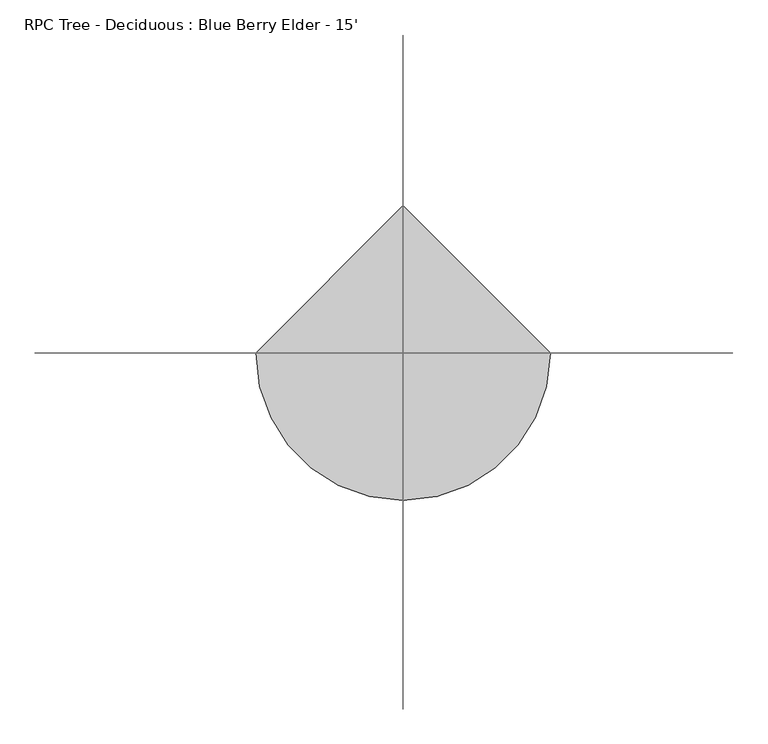
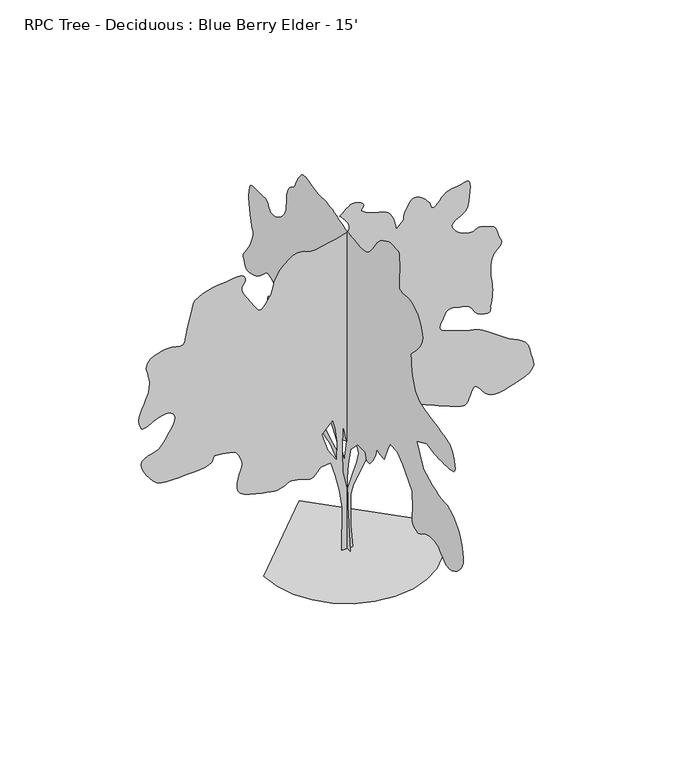
"""IFC4 building model written with IfcOpenShell, lengths in millimetres: geographic element geometry, RPC Tree - Deciduous : Blue Berry Elder - 15'."""

from ifc_helpers import new_model, si_unit, origin, place, context, project, spatial, triangles, source, transform, mapped, element, save


def rpc_tree_deciduous_blue_berry_elder_15_4a646840(model_context):
    return source(origin(), model_context, "Body", "Tessellation", [
        triangles([(-0.0006962, 27.8334278, 0.0019603), (-0.0006962, -29.6324096, 0.0019603), (-0.0006962, -7.2846616, 268.1759455), (-0.0006962, -0.8995193, 430.9958582), (-0.0006962, -10.4771573, 523.5799235), (-0.0006962, -36.0175667, 628.9336309), (-0.0006962, -106.2537161, 699.1706228), (-0.0006962, -179.6824553, 699.1706228), (-0.0006962, -195.6453436, 654.4740051), (-0.0006962, -227.5699575, 657.6673422), (-0.0006962, -262.6890348, 699.1706228), (-0.0006962, -285.0361446, 743.8660051), (-0.0006962, -297.8069494, 788.5613874), (-0.0006962, -332.9248458, 775.791818), (-0.0006962, -371.2348257, 772.598481), (-0.0006962, -406.3527403, 852.4130133), (-0.0006962, -431.8931508, 900.3004972), (-0.0006962, -502.1301064, 897.1083956), (-0.0006962, -556.4030291, 852.4130133), (-0.0006962, -655.3724968, 747.0581068), (-0.0006962, -658.5645985, 641.7044357), (-0.0006962, -657.5866785, 629.1849237), (-0.0006962, -655.4376818, 614.2651222), (-0.0006962, -653.2875223, 598.0604064), (-0.0006962, -652.3096024, 581.6873869), (-0.0006962, -653.6774694, 566.2649998), (-0.0006962, -658.5645985, 552.9086566), (-0.0006962, -668.1421389, 542.7349317), (-0.0006962, -680.1305786, 535.3822918), (-0.0006962, -691.7279085, 530.0388316), (-0.0006962, -703.3252384, 527.1537243), (-0.0006962, -715.3136782, 527.1726912), (-0.0006962, -728.084483, 530.5425799), (-0.0006962, -742.0263645, 537.709112), (-0.0006962, -757.5340662, 549.1203341), (-0.0006962, -776.7637791, 561.2296967), (-0.0006962, -800.3495487, 570.1552783), (-0.0006962, -826.3925085, 575.8425038), (-0.0006962, -852.9937918, 578.234509), (-0.0006962, -878.2544592, 577.276755), (-0.0006962, -900.2768068, 572.9111784), (-0.0006962, -917.1607327, 565.0832405), (-0.0006962, -931.1227438, 553.3365738), (-0.0006962, -945.9773603, 538.7427335), (-0.0006962, -962.2282579, 523.5337054), (-0.0006962, -980.3793303, 509.9438373), (-0.0006962, -1000.9306194, 500.208712), (-0.0006962, -1024.3860191, 496.5590438), (-0.0006962, -1051.248115, 501.231651), (-0.0006962, -1078.7241268, 513.6764583), (-0.0006962, -1103.3530014, 530.8116405), (-0.0006962, -1124.629755, 551.0749386), (-0.0006962, -1142.0542002, 572.901695), (-0.0006962, -1155.1225159, 594.7284513), (-0.0006962, -1163.3309538, 614.990514), (-0.0006962, -1166.1792538, 632.1268953), (-0.0006962, -1164.3550192, 650.8540226), (-0.0006962, -1159.4039406, 675.2209219), (-0.0006962, -1152.1058395, 702.6602354), (-0.0006962, -1143.2454065, 730.6021345), (-0.0006962, -1133.6027538, 756.4779533), (-0.0006962, -1123.9600285, 777.7180086), (-0.0006962, -1115.0985054, 791.7534891), (-0.0006962, -1104.8050203, 803.3887527), (-0.0006962, -1090.6011635, 817.9825567), (-0.0006962, -1072.8792801, 833.8068089), (-0.0006962, -1052.0304073, 849.12724), (-0.0006962, -1028.4446377, 862.2133598), (-0.0006962, -1002.513081, 871.3344601), (-0.0006962, -974.6269197, 874.7601231), (-0.0006962, -945.6146645, 877.0869432), (-0.0006962, -916.0998236, 883.6026793), (-0.0006962, -886.1665489, 893.6081005), (-0.0006962, -855.8979023, 906.4061565), (-0.0006962, -825.3778902, 921.2987068), (-0.0006962, -794.6895744, 937.5875381), (-0.0006962, -763.9183422, 954.57342), (-0.0006962, -696.8746147, 1079.0832619), (-0.0006962, -799.0361841, 1126.9719812), (-0.0006962, -812.7931932, 1122.8943958), (-0.0006962, -826.9970501, 1118.9851868), (-0.0006962, -842.0946751, 1115.4114223), (-0.0006962, -858.5316805, 1112.3402435), (-0.0006962, -876.7562222, 1109.9387186), (-0.0006962, -897.2150751, 1108.3752966), (-0.0006962, -920.353997, 1107.8158104), (-0.0006962, -946.7881393, 1107.7138544), (-0.0006962, -975.4554302, 1107.7790394), (-0.0006962, -1004.2910975, 1108.5696888), (-0.0006962, -1031.2277527, 1110.6463789), (-0.0006962, -1054.1983709, 1114.5638723), (-0.0006962, -1071.1391973, 1120.8841261), (-0.0006962, -1079.9805908, 1130.1640829), (-0.0006962, -1081.6756182, 1144.7863735), (-0.0006962, -1079.0690912, 1165.0496716), (-0.0006962, -1072.9444651, 1188.3805876), (-0.0006962, -1064.0828693, 1212.21765), (-0.0006962, -1053.2679045, 1233.9922657), (-0.0006962, -1041.2793921, 1251.1322079), (-0.0006962, -1028.8997698, 1261.0534046), (-0.0006962, -1016.4087444, 1266.0318798), (-0.0006962, -1002.85681, 1270.3346695), (-0.0006962, -987.1831301, 1274.4595631), (-0.0006962, -968.3256329, 1278.928331), (-0.0006962, -945.2234819, 1284.2386173), (-0.0006962, -916.8157682, 1290.8764389), (-0.0006962, -882.0428181, 1299.3634209), (-0.0006962, -844.7746714, 1307.803022), (-0.0006962, -809.8523844, 1314.8438713), (-0.0006962, -777.6658316, 1321.8136494), (-0.0006962, -748.6073582, 1330.0872723), (-0.0006962, -723.066984, 1340.9805027), (-0.0006962, -701.4358189, 1355.8327938), (-0.0006962, -684.1050453, 1375.9953712), (-0.0006962, -670.8233706, 1400.3658314), (-0.0006962, -660.7242777, 1426.7512848), (-0.0006962, -653.2780025, 1454.8200657), (-0.0006962, -647.9534729, 1484.2163818), (-0.0006962, -644.2208519, 1514.6319672), (-0.0006962, -641.5503027, 1545.7114655), (-0.0006962, -639.4095903, 1577.1227749), (-0.0006962, -663.2087191, 1601.7422024), (-0.0006962, -686.1438017, 1626.3023312), (-0.0006962, -707.3458506, 1650.7557804), (-0.0006962, -725.952055, 1675.0432514), (-0.0006962, -741.0958981, 1699.0936729), (-0.0006962, -751.9120256, 1722.8833546), (-0.0006962, -757.5340662, 1746.3293072), (-0.0006962, -755.6351995, 1772.2525795), (-0.0006962, -745.4709217, 1801.6369778), (-0.0006962, -728.5491348, 1831.6851437), (-0.0006962, -706.3786131, 1859.6235546), (-0.0006962, -680.4660233, 1882.6427891), (-0.0006962, -652.3191221, 1897.9453434), (-0.0006962, -623.4466839, 1902.7578403), (-0.0006962, -596.6771333, 1901.3236256), (-0.0006962, -573.873656, 1900.2094494), (-0.0006962, -555.0908635, 1900.1619232), (-0.0006962, -540.3844211, 1901.9044041), (-0.0006962, -529.8112292, 1906.1598129), (-0.0006962, -523.4258268, 1913.6510708), (-0.0006962, -521.2851145, 1925.1133072), (-0.0006962, -522.0946944, 1946.4848225), (-0.0006962, -523.853744, 1979.579314), (-0.0006962, -525.5570558, 2018.9324352), (-0.0006962, -526.1995311, 2059.0679214), (-0.0006962, -524.7747634, 2094.5093628), (-0.0006962, -520.2799796, 2119.7925579), (-0.0006962, -511.7076104, 2129.4293243), (-0.0006962, -499.1608472, 2130.0813194), (-0.0006962, -484.0442917, 2131.5155342), (-0.0006962, -467.309739, 2132.949749), (-0.0006962, -449.9042971, 2133.6017441), (-0.0006962, -432.7773992, 2132.6890091), (-0.0006962, -416.879714, 2129.4293243), (-0.0006962, -403.1606386, 2123.0522427), (-0.0006962, -390.1302567, 2115.4660778), (-0.0006962, -375.9263998, 2108.5675163), (-0.0006962, -360.9402143, 2101.43176), (-0.0006962, -345.5640452, 2093.1818275), (-0.0006962, -330.1879126, 2082.9286743), (-0.0006962, -315.2028897, 2069.7714832), (-0.0006962, -300.999051, 2052.8092918), (-0.0006962, -286.7584414, 2032.3385937), (-0.0006962, -271.5126786, 2010.2557846), (-0.0006962, -255.4288675, 1988.0545235), (-0.0006962, -238.6741671, 1967.2518688), (-0.0006962, -221.4180801, 1949.3533974), (-0.0006962, -203.8265303, 1935.8642498), (-0.0006962, -186.0678577, 1928.3017754), (-0.0006962, -167.8895705, 1925.4688087), (-0.0006962, -148.9301446, 1924.816959), (-0.0006962, -129.188399, 1925.7888474), (-0.0006962, -108.6643338, 1927.8157585), (-0.0006962, -87.3590209, 1930.3523769), (-0.0006962, -65.2717381, 1932.829842), (-0.0006962, -42.4027261, 1934.6907749), (-0.0006962, -15.4102944, 1938.1638187), (-0.0006962, 16.7757986, 1944.9439281), (-0.0006962, 50.749019, 1953.6205788), (-0.0006962, 83.1026037, 1962.7950188), (-0.0006962, 110.4301236, 1971.0805595), (-0.0006962, 129.3247097, 1977.0783039), (-0.0006962, 136.3798205, 1979.3778728), (-0.0006962, 140.2617874, 1980.586956), (-0.0006962, 151.0115855, 1983.5857555), (-0.0006962, 167.2909697, 1987.4262188), (-0.0006962, 187.7581434, 1991.14823), (-0.0006962, 211.0748524, 1993.8034458), (-0.0006962, 235.8981192, 1994.4552956), (-0.0006962, 260.8897079, 1992.1557266), (-0.0006962, 288.430941, 1991.7053181), (-0.0006962, 320.1611627, 1996.7904728), (-0.0006962, 353.6219473, 2004.7203667), (-0.0006962, 386.3573401, 2012.8160934), (-0.0006962, 415.9100784, 2018.3990376), (-0.0006962, 439.8206466, 2018.7902927), (-0.0006962, 455.6353789, 2011.3108074), (-0.0006962, 466.5440154, 1998.4499645), (-0.0006962, 477.2286103, 1984.6288605), (-0.0006962, 487.4675202, 1970.0967533), (-0.0006962, 497.0355409, 1955.0547935), (-0.0006962, 505.7098297, 1939.7284035), (-0.0006962, 513.268707, 1924.3546326), (-0.0006962, 519.4858057, 1909.1468399), (-0.0006962, 526.9130776, 1896.1673996), (-0.0006962, 537.4685017, 1886.2698933), (-0.0006962, 549.9773312, 1877.8183743), (-0.0006962, 563.2696521, 1869.2010223), (-0.0006962, 576.1696641, 1858.7938087), (-0.0006962, 587.5061814, 1844.97285), (-0.0006962, 596.1069646, 1826.1378078), (-0.0006962, 601.3283755, 1809.8395294), (-0.0006962, 603.8697175, 1802.0873863), (-0.0006962, 604.5678944, 1798.9106907), (-0.0006962, 604.2609, 1796.3503819), (-0.0006962, 603.7855657, 1790.4473991), (-0.0006962, 603.9811569, 1777.2191368), (-0.0006962, 605.6844687, 1752.7063889), (-0.0006962, 608.6916615, 1724.7088245), (-0.0006962, 612.535722, 1702.6970867), (-0.0006962, 617.6634613, 1685.1897251), (-0.0006962, 624.522999, 1670.7642975), (-0.0006962, 633.5611828, 1657.962608), (-0.0006962, 645.2236977, 1645.3151241), (-0.0006962, 659.9585541, 1631.3992584), (-0.0006962, 676.6931431, 1617.5426914), (-0.0006962, 693.7642668, 1606.2109703), (-0.0006962, 710.7216619, 1597.5460922), (-0.0006962, 727.121969, 1591.7380165), (-0.0006962, 742.5171049, 1588.9524307), (-0.0006962, 756.4602219, 1589.3436859), (-0.0006962, 768.5043995, 1593.0892422), (-0.0006962, 777.4406273, 1600.4383575), (-0.0006962, 783.6944607, 1610.4662338), (-0.0006962, 789.2797302, 1621.5610508), (-0.0006962, 796.2044529, 1632.0986343), (-0.0006962, 806.4801338, 1640.4552464), (-0.0006962, 822.1170427, 1645.0187759), (-0.0006962, 845.1255947, 1644.1653397), (-0.0006962, 872.6667915, 1642.5058479), (-0.0006962, 899.7066381, 1643.8096928), (-0.0006962, 924.9578585, 1645.1728363), (-0.0006962, 947.13899, 1643.6793228), (-0.0006962, 964.9628294, 1636.436887), (-0.0006962, 977.1468967, 1620.5416363), (-0.0006962, 982.4050787, 1593.0892422), (-0.0006962, 983.5406199, 1565.7080647), (-0.0006962, 984.0621723, 1548.8288624), (-0.0006962, 983.7456945, 1537.7105003), (-0.0006962, 982.3683077, 1527.5994896), (-0.0006962, 979.7060429, 1513.7311501), (-0.0006962, 975.5360212, 1491.3876011), (-0.0006962, 969.6354366, 1455.8038719), (-0.0006962, 961.9189018, 1419.4496956), (-0.0006962, 953.6452789, 1394.8183502), (-0.0006962, 946.5984707, 1377.2279995), (-0.0006962, 942.5683388, 1361.9845985), (-0.0006962, 943.341184, 1344.3942478), (-0.0006962, 950.7033073, 1319.7630478), (-0.0006962, 966.4421722, 1283.4088715), (-0.0006962, 986.743404, 1245.2885239), (-0.0006962, 1005.7027845, 1216.9471579), (-0.0006962, 1021.9821688, 1196.0378237), (-0.0006962, 1034.2397055, 1180.2029617), (-0.0006962, 1041.1371769, 1167.1062321), (-0.0006962, 1041.3327318, 1154.401775), (-0.0006962, 1033.4858271, 1139.7415506), (-0.0006962, 1024.3362402, 1124.5610092), (-0.0006962, 1019.3199039, 1112.116202), (-0.0006962, 1015.1404352, 1102.7994741), (-0.0006962, 1008.5037764, 1097.0007729), (-0.0006962, 996.115797, 1095.1113533), (-0.0006962, 974.6802595, 1097.5223253), (-0.0006962, 940.9017254, 1104.6237087), (-0.0006962, 904.0438007, 1118.2964933), (-0.0006962, 874.3334049, 1137.777499), (-0.0006962, 849.9285719, 1159.492816), (-0.0006962, 828.9860275, 1179.8675171), (-0.0006962, 809.6639511, 1195.3266752), (-0.0006962, 790.1165977, 1202.2963806), (-0.0006962, 768.5043995, 1197.2112986), (-0.0006962, 747.6649738, 1185.1730799), (-0.0006962, 731.1805876, 1173.6409349), (-0.0006962, 718.3267937, 1162.5272964), (-0.0006962, 708.3771103, 1151.7490299), (-0.0006962, 700.6048376, 1141.2220562), (-0.0006962, 694.2846565, 1130.8622234), (-0.0006962, 688.6911026, 1120.5866152), (-0.0006962, 697.5798769, 1111.7345392), (-0.0006962, 706.4402372, 1103.1349188), (-0.0006962, 715.2460951, 1095.0367212), (-0.0006962, 723.9666384, 1087.6935648), (-0.0006962, 732.5768686, 1081.3544168), (-0.0006962, 741.0472818, 1076.2728956), (-0.0006962, 749.3493914, 1072.6978958), (-0.0006962, 758.2014673, 1071.0787359), (-0.0006962, 767.7789351, 1070.6875534), (-0.0006962, 777.2449997, 1070.0178268), (-0.0006962, 785.761631, 1067.5606367), (-0.0006962, 792.4907988, 1061.8082262), (-0.0006962, 796.5956354, 1051.2528385), (-0.0006962, 797.2380381, 1034.3878796), (-0.0006962, 795.1151299, 1015.5861202), (-0.0006962, 791.5970306, 999.2972162), (-0.0006962, 786.8497913, 984.1261219), (-0.0006962, 781.041643, 968.6753208), (-0.0006962, 774.3409618, 951.5484592), (-0.0006962, 766.9124908, 931.3515089), (-0.0006962, 758.9268591, 906.6858633), (-0.0006962, 750.6804874, 878.9206249), (-0.0006962, 742.9924393, 851.0996487), (-0.0006962, 736.8120752, 824.3407442), (-0.0006962, 733.088974, 799.7580877), (-0.0006962, 732.7724962, 778.4718143), (-0.0006962, 736.8120752, 761.5974083), (-0.0006962, 746.1572897, 750.2513712), (-0.0006962, 758.1919476, 742.6925303), (-0.0006962, 769.7240925, 736.3083269), (-0.0006962, 780.8378036, 730.8996454), (-0.0006962, 791.6159975, 726.2744917), (-0.0006962, 802.1429712, 722.23484), (-0.0006962, 812.502804, 718.5863708), (-0.0006962, 822.7784849, 715.1322939), (-0.0006962, 833.6396679, 719.758683), (-0.0006962, 843.9995007, 723.4071522), (-0.0006962, 853.3541622, 725.1010168), (-0.0006962, 861.1999043, 723.8635197), (-0.0006962, 867.0364666, 718.7167408), (-0.0006962, 870.3589382, 708.6829056), (-0.0006962, 870.6659689, 692.7851841), (-0.0006962, 867.9017481, 675.8633972), (-0.0006962, 862.6246719, 662.9633852), (-0.0006962, 855.2530289, 653.4131687), (-0.0006962, 846.205398, 646.5441113), (-0.0006962, 835.9013031, 641.6854689), (-0.0006962, 824.7603407, 638.1673697), (-0.0006962, 813.1997818, 635.318997), (-0.0006962, 807.717631, 631.8471886), (-0.0006962, 802.1797422, 628.0683495), (-0.0006962, 796.5303778, 623.6755217), (-0.0006962, 790.7127823, 618.3604391), (-0.0006962, 784.672308, 611.8173792), (-0.0006962, 778.3521269, 603.7381485), (-0.0006962, 771.6976639, 593.8157164), (-0.0006962, 762.5291101, 583.2425609), (-0.0006962, 749.1727306, 573.3390956), (-0.0006962, 732.3255758, 563.9939175), (-0.0006962, 712.6857862, 555.0955871), (-0.0006962, 690.9526651, 546.5327376), (-0.0006962, 667.823263, 538.1927307), (-0.0006962, 643.9956476, 529.9653259), (-0.0006962, 567.3744887, 574.6607446), (-0.0006962, 490.7532935, 517.1945211), (-0.0006962, 480.5049002, 515.8633887), (-0.0006962, 470.3406587, 514.7562979), (-0.0006962, 460.3447208, 514.094892), (-0.0006962, 450.5989131, 514.1043755), (-0.0006962, 441.1897127, 515.0075907), (-0.0006962, 432.1977834, 517.0274165), (-0.0006962, 423.7096024, 520.3878219), (-0.0006962, 415.83541, 524.8363875), (-0.0006962, 408.406939, 529.7875388), (-0.0006962, 401.0910338, 534.9626953), (-0.0006962, 393.5523225, 540.0821503), (-0.0006962, 385.4541249, 544.8661606), (-0.0006962, 376.4633583, 549.0361822), (-0.0006962, 366.2434153, 552.3124357), (-0.0006962, 354.7397206, 554.8632611), (-0.0006962, 342.2297284, 557.0786782), (-0.0006962, 328.8828323, 559.0143159), (-0.0006962, 314.8650833, 560.7271111), (-0.0006962, 300.3447487, 562.2716025), (-0.0006962, 285.4901321, 563.7058537), (-0.0006962, 270.4672119, 565.0832405), (-0.0006962, 171.497726, 536.3495293), (-0.0006962, 88.491846, 475.6912405), (-0.0006962, 43.7962048, 402.263346), (-0.0006962, 21.4482684, 261.7905613), (-0.0006523, 31.0258883, 520.3878219), (-0.0006523, 78.9142239, 622.5494276), (-0.0006523, 2.2929818, 654.4740051), (-0.0006582, 145.9573246, 555.5057364), (-0.0006582, 222.5785107, 606.5865211), (-0.0006582, 283.2368176, 609.7786228), (-0.0006582, 334.3176023, 638.5110987), (-0.0006582, 331.5629013, 639.9916042), (-0.0006582, 328.6955618, 642.1418364), (-0.0006582, 325.6065788, 645.6326117), (-0.0006582, 322.1809522, 651.1325666), (-0.0006582, 318.3084778, 659.314916), (-0.0006582, 313.878879, 670.847061), (-0.0006582, 308.7771918, 686.399818), (-0.0006582, 304.7008418, 701.7664673), (-0.0006582, 303.1373835, 712.7782225), (-0.0006582, 303.6672385, 720.1593126), (-0.0006582, 305.873154, 724.6363649), (-0.0006582, 309.336678, 726.9346985), (-0.0006582, 313.6359069, 727.7821758), (-0.0006582, 318.3558949, 727.9030987), (-0.0006582, 321.5479966, 766.2131149), (-0.0006582, 283.2368176, 791.7534891), (-0.0006582, 200.2314009, 721.5177326), (-0.0006582, 142.7652138, 654.4740051), (-0.0006582, 104.4544981, 600.2011188), (-0.0006582, 66.1439051, 514.0024195), (31.5943742, 0.0001246, 0.0), (-32.2567384, 0.0001246, 0.0), (-29.0642779, 0.0001077, 261.7893804), (-45.0270572, 0.0001014, 376.7205737), (-67.3747574, 9.51e-05, 472.4967771), (-96.1076148, 9.08e-05, 558.6954763), (-153.5730934, 9.08e-05, 552.3112367), (-163.1790477, 9.08e-05, 538.7676229), (-172.9521249, 9.29e-05, 526.0632022), (-183.0606648, 9.29e-05, 515.0336792), (-193.6717722, 9.29e-05, 506.5170479), (-204.952588, 9.51e-05, 501.3513748), (-217.0702713, 9.51e-05, 500.3734549), (-230.1942886, 9.29e-05, 504.4225536), (-244.1563361, 9.29e-05, 510.5187295), (-258.6209692, 9.29e-05, 515.2754886), (-273.504036, 9.29e-05, 518.9144743), (-288.7213484, 9.29e-05, 521.660891), (-304.1911527, 9.29e-05, 523.736382), (-319.8280798, 9.29e-05, 525.3650617), (-335.5491769, 9.29e-05, 526.7708625), (-348.5890423, 9.29e-05, 519.3245873), (-361.8802005, 9.29e-05, 512.3524475), (-375.675107, 9.29e-05, 506.3309401), (-390.2227292, 9.29e-05, 501.7330376), (-405.7754863, 9.51e-05, 499.0340381), (-422.5859064, 9.51e-05, 498.7080769), (-440.902848, 9.51e-05, 501.230452), (-464.5822892, 9.29e-05, 505.7999042), (-495.0738147, 9.29e-05, 511.5985691), (-529.0289005, 9.29e-05, 519.0732945), (-563.0954258, 9.29e-05, 528.6697655), (-593.9223959, 9.08e-05, 540.8348296), (-618.1589252, 9.08e-05, 556.0154074), (-632.455291, 8.87e-05, 574.6583465), (-637.0721603, 8.87e-05, 596.876249), (-635.7694782, 8.66e-05, 621.4387396), (-630.4449486, 8.45e-05, 646.7847942), (-622.9986734, 8.45e-05, 671.3472485), (-615.3295195, 8.24e-05, 693.565151), (-609.3352996, 8.24e-05, 711.8726818), (-606.9148441, 8.03e-05, 724.7086716), (-608.023134, 8.03e-05, 735.682493), (-611.0848658, 8.03e-05, 748.77806), (-615.7112549, 7.82e-05, 762.9913639), (-621.5098835, 7.82e-05, 777.3161436), (-628.0908772, 7.6e-05, 790.7471552), (-635.0618179, 7.6e-05, 802.2793001), (-642.0339214, 7.6e-05, 810.9073345), (-651.2013124, 7.6e-05, 817.0971457), (-664.5588547, 7.39e-05, 822.1134819), (-681.4048468, 7.39e-05, 826.1531336), (-701.0446363, 7.39e-05, 829.4104202), (-722.7777575, 7.39e-05, 832.0821321), (-745.9071596, 7.39e-05, 834.3627342), (-769.734775, 7.39e-05, 836.4477087), (-773.4400721, 7.39e-05, 824.2174232), (-778.8475908, 7.6e-05, 812.4897234), (-787.6617331, 7.6e-05, 801.7671947), (-801.5870459, 7.6e-05, 792.5524229), (-822.3244429, 7.6e-05, 785.3479935), (-851.5785439, 7.82e-05, 780.6575821), (-891.0525152, 7.82e-05, 778.9815216), (-934.7890171, 7.82e-05, 777.8921986), (-975.5111681, 7.82e-05, 775.7420391), (-1012.9368633, 7.82e-05, 774.2070311), (-1046.7888668, 7.82e-05, 774.9609095), (-1076.7884892, 7.82e-05, 779.6797348), (-1102.6536255, 7.6e-05, 790.0394949), (-1124.1082026, 7.6e-05, 807.7152328), (-1143.5156662, 7.39e-05, 830.946591), (-1162.0839369, 7.39e-05, 855.9654127), (-1177.8050703, 7.18e-05, 881.4323175), (-1188.6650906, 6.97e-05, 906.0043642), (-1192.6596142, 6.76e-05, 928.343117), (-1187.776046, 6.76e-05, 947.1070152), (-1171.9969219, 6.76e-05, 960.9564606), (-1151.4171461, 6.55e-05, 969.659127), (-1133.2388226, 6.55e-05, 975.0678085), (-1117.127742, 6.55e-05, 978.9675705), (-1102.7472971, 6.55e-05, 983.1470392), (-1089.7631332, 6.55e-05, 989.3925882), (-1077.8398785, 6.34e-05, 999.4904457), (-1066.6420155, 6.34e-05, 1015.230546), (-1053.3888273, 6.13e-05, 1035.9584232), (-1037.2302933, 6.13e-05, 1059.0878981), (-1020.7363873, 5.91e-05, 1083.5021782), (-1006.4767925, 5.7e-05, 1108.083672), (-997.0202477, 5.7e-05, 1131.7168951), (-994.9352005, 5.49e-05, 1153.2828753), (-1002.791625, 5.49e-05, 1171.6650381), (-1017.218288, 5.28e-05, 1184.6396822), (-1032.9856396, 5.28e-05, 1191.4150681), (-1049.8695654, 5.28e-05, 1193.0271063), (-1067.6471867, 5.28e-05, 1190.5023331), (-1086.0956972, 5.28e-05, 1184.8826906), (-1104.9899654, 5.28e-05, 1177.1934071), (-1124.1082026, 5.49e-05, 1168.4729364), (-1137.7158749, 5.49e-05, 1161.0633596), (-1150.8777895, 5.49e-05, 1154.3532314), (-1163.144846, 5.49e-05, 1149.0381489), (-1174.0712139, 5.49e-05, 1145.8176332), (-1183.2125164, 5.49e-05, 1145.3896797), (-1190.1230684, 5.49e-05, 1148.4514114), (-1194.3427963, 5.49e-05, 1155.7021317), (-1197.5313372, 5.49e-05, 1164.6845776), (-1201.0518345, 5.49e-05, 1173.2201757), (-1204.0625519, 5.28e-05, 1182.4255005), (-1205.7338888, 5.28e-05, 1193.4182888), (-1205.2360268, 5.28e-05, 1207.3103914), (-1201.7156021, 5.07e-05, 1225.232626), (-1194.3427963, 4.86e-05, 1248.2873234), (-1184.4785002, 4.86e-05, 1272.8830605), (-1174.4445923, 4.65e-05, 1295.3688972), (-1164.8576048, 4.65e-05, 1316.72864), (-1156.3315264, 4.44e-05, 1337.9697853), (-1149.4815084, 4.22e-05, 1360.1236656), (-1144.9203043, 4.22e-05, 1384.1623146), (-1143.2632107, 4.01e-05, 1411.1048561), (-1145.1348261, 3.8e-05, 1436.9451393), (-1149.6296099, 3.8e-05, 1457.9255447), (-1155.0750624, 3.59e-05, 1475.4448242), (-1159.7938877, 3.59e-05, 1490.8898117), (-1162.1124235, 3.38e-05, 1505.6708862), (-1160.3522112, 3.38e-05, 1521.1750271), (-1152.8419138, 3.17e-05, 1538.8127586), (-1138.7032419, 3.17e-05, 1555.7038788), (-1119.4830488, 2.96e-05, 1568.4106613), (-1097.1347763, 2.96e-05, 1577.431041), (-1073.614119, 2.96e-05, 1583.2628071), (-1050.8758993, 2.96e-05, 1586.4158123), (-1030.8733412, 2.96e-05, 1587.3996185), (-1015.5624298, 2.96e-05, 1586.700388), (-1002.4289291, 2.96e-05, 1584.0807804), (-988.2902573, 2.96e-05, 1580.2403172), (-974.0958475, 2.96e-05, 1577.0636215), (-960.7952059, 2.96e-05, 1576.4590073), (-949.336603, 2.96e-05, 1580.3231609), (-940.6717976, 2.96e-05, 1590.5526237), (-935.7478975, 2.75e-05, 1609.0439369), (-931.5873957, 2.53e-05, 1635.7731194), (-925.1368446, 2.53e-05, 1667.7060539), (-917.2353647, 2.32e-05, 1702.1992973), (-908.7187334, 2.11e-05, 1736.633242), (-900.4249809, 1.9e-05, 1768.3884258), (-893.1932276, 1.69e-05, 1794.8449505), (-887.8592508, 1.48e-05, 1813.3717266), (-878.3374483, 1.48e-05, 1826.7778851), (-859.7691776, 1.48e-05, 1839.3542976), (-834.8332724, 1.27e-05, 1850.6505558), (-806.2121996, 1.27e-05, 1860.2043331), (-776.5859556, 1.27e-05, 1867.5890568), (-748.6346094, 1.27e-05, 1872.3421097), (-725.03932, 1.27e-05, 1874.0252918), (-703.0360119, 1.27e-05, 1875.6610931), (-679.1894297, 1.27e-05, 1879.3118877), (-655.1757792, 1.27e-05, 1883.0695072), (-632.6698128, 1.06e-05, 1885.0488922), (-613.346501, 1.27e-05, 1883.3302471), (-598.8830306, 1.27e-05, 1876.0404305), (-590.951974, 1.27e-05, 1861.2593559), (-590.7575818, 1.48e-05, 1844.97285), (-596.034658, 1.48e-05, 1832.6571774), (-603.2664113, 1.48e-05, 1821.633577), (-608.935869, 1.69e-05, 1809.2112247), (-609.5214074, 1.69e-05, 1792.6995872), (-601.5073617, 1.9e-05, 1769.4433033), (-581.3756327, 2.11e-05, 1736.7518394), (-557.4639018, 2.32e-05, 1701.8081875), (-539.4159845, 2.32e-05, 1673.7867874), (-525.6684952, 2.53e-05, 1652.9723602), (-514.6579391, 2.53e-05, 1639.6491909), (-504.8196588, 2.75e-05, 1634.0781647), (-494.5901959, 2.53e-05, 1636.5554844), (-482.4061649, 2.53e-05, 1647.3538078), (-469.5061529, 2.53e-05, 1662.9528557), (-458.1684365, 2.32e-05, 1679.5001015), (-448.3953775, 2.32e-05, 1696.7823315), (-440.1869396, 2.11e-05, 1714.5623508), (-433.540761, 2.11e-05, 1732.615028), (-428.4592398, 1.9e-05, 1750.7268585), (-424.9399778, 1.9e-05, 1768.6728561), (-418.4988739, 1.69e-05, 1789.3569134), (-405.4684919, 1.48e-05, 1814.1067108), (-387.0768456, 1.48e-05, 1840.3737122), (-364.5519124, 1.27e-05, 1865.585836), (-339.1229413, 1.06e-05, 1887.1587925), (-312.0191088, 1.06e-05, 1902.5327087), (-284.468374, 1.06e-05, 1909.1468399), (-262.1105999, 1.06e-05, 1908.2814857), (-247.1255952, 1.06e-05, 1904.1683647), (-235.5460695, 1.06e-05, 1898.6684097), (-223.4094375, 1.06e-05, 1893.6188633), (-206.7483723, 1.06e-05, 1890.8571133), (-181.5991443, 1.06e-05, 1892.2202568), (-143.9955984, 1.06e-05, 1899.5693722), (-101.8225821, 1.06e-05, 1909.134922), (-65.7924549, 1.06e-05, 1916.6973965), (-36.1845805, 8.4e-06, 1923.3589085), (-13.2783513, 8.4e-06, 1930.2456974), (2.6471004, 8.4e-06, 1938.4719395), (11.3125692, 8.4e-06, 1949.1518108), (12.438779, 6.3e-06, 1963.4114056), (8.6785434, 6.3e-06, 1978.9037739), (3.0753261, 4.2e-06, 1992.7128147), (-4.0636578, 4.2e-06, 2005.1351669), (-12.4313122, 4.2e-06, 2016.4314251), (-21.7203017, 2.1e-06, 2026.8979374), (-31.6236511, 2.1e-06, 2036.7954437), (-41.8342379, 2.1e-06, 2046.4204376), (-28.8685799, 2.1e-06, 2058.6412033), (-16.0983803, 0.0, 2070.3048809), (-3.7191759, 0.0, 2080.8543823), (8.0736913, 0.0, 2089.7207016), (19.0847113, 0.0, 2096.3585232), (29.1184488, -2.1e-06, 2100.1989864), (37.9794132, -2.1e-06, 2100.6967758), (47.1939671, -2.1e-06, 2098.918832), (57.7490141, 0.0, 2096.2518436), (68.6389154, 0.0, 2092.5654408), (78.8588675, 0.0, 2087.7766342), (87.4033496, 0.0, 2081.7551994), (93.2671995, 0.0, 2074.3943115), (95.4452461, 0.0, 2065.5753731), (93.4626636, 2.1e-06, 2057.574408), (88.9670441, 2.1e-06, 2051.9677734), (84.1364523, 2.1e-06, 2047.6530659), (81.1486987, 2.1e-06, 2043.5044819), (82.1818296, 2.1e-06, 2038.3956367), (89.41391, 2.1e-06, 2031.23619), (105.0229863, 4.2e-06, 2020.8882751), (126.0211868, 4.2e-06, 2010.3506916), (147.5219638, 4.2e-06, 2002.6578472), (168.8556089, 4.2e-06, 1996.7548645), (189.3512329, 4.2e-06, 1991.586866), (208.3391001, 6.3e-06, 1986.0749931), (225.1483212, 6.3e-06, 1979.1645138), (239.1103686, 6.3e-06, 1969.8004051), (250.2145782, 6.3e-06, 1957.7336998), (259.1401598, 8.4e-06, 1943.6637737), (266.2509722, 8.4e-06, 1927.922438), (271.9097656, 1.06e-05, 1910.830022), (276.4803987, 1.06e-05, 1892.7299641), (280.3244409, 1.27e-05, 1873.9661385), (283.8057691, 1.27e-05, 1854.8703564), (328.5011696, 1.06e-05, 1896.3688408), (328.2036587, 1.06e-05, 1898.0520229), (327.6821062, 1.06e-05, 1902.7460678), (327.4959984, 1.06e-05, 1909.9409775), (328.2036587, 1.06e-05, 1919.1629436), (330.3633379, 8.4e-06, 1929.878278), (334.5333232, 8.4e-06, 1941.6131721), (341.2719744, 8.4e-06, 1953.8339378), (348.9967936, 6.3e-06, 1966.5644108), (356.1644883, 6.3e-06, 1979.4015633), (363.3867582, 4.2e-06, 1991.2785999), (371.2798811, 4.2e-06, 2001.1643337), (380.4567555, 4.2e-06, 2007.9681335), (391.5324966, 4.2e-06, 2010.6351219), (405.1223648, 4.2e-06, 2008.1104214), (419.2420698, 4.2e-06, 2001.9940796), (431.6868771, 4.2e-06, 1994.692345), (442.7354033, 6.3e-06, 1986.4187222), (452.6661198, 6.3e-06, 1977.3627342), (461.7600051, 6.3e-06, 1967.7141953), (470.2944042, 6.3e-06, 1957.6861736), (478.5514584, 8.4e-06, 1947.4568562), (480.6637204, 8.4e-06, 1937.322155), (483.1398774, 8.4e-06, 1927.9343559), (486.3414625, 8.4e-06, 1920.0637608), (490.6323707, 1.06e-05, 1914.4452084), (496.3753341, 1.06e-05, 1911.8494366), (503.9330123, 1.06e-05, 1913.0229115), (513.6693366, 1.06e-05, 1918.7243076), (524.3456471, 8.4e-06, 1928.6455044), (534.9650571, 8.4e-06, 1941.0204758), (546.2553926, 8.4e-06, 1954.4027985), (558.9420093, 6.3e-06, 1967.3467758), (573.7504077, 6.3e-06, 1978.3821487), (591.4071424, 6.3e-06, 1986.0749931), (612.637678, 6.3e-06, 1988.9553406), (635.5442739, 4.2e-06, 1991.3971973), (657.1101814, 4.2e-06, 1996.7429466), (676.3861124, 4.2e-06, 2002.0295425), (692.4237236, 4.2e-06, 2004.2936485), (704.2722736, 4.2e-06, 2000.5953278), (710.9836372, 6.3e-06, 1987.9478439), (711.6071457, 6.3e-06, 1963.4114056), (709.3170965, 8.4e-06, 1933.3395493), (707.362492, 1.06e-05, 1906.1005142), (704.9052292, 1.27e-05, 1881.8248158), (701.1086586, 1.27e-05, 1860.6192787), (695.1322065, 1.48e-05, 1842.6022099), (686.1414036, 1.48e-05, 1827.8802887), (673.2971294, 1.48e-05, 1816.5603401), (657.2216572, 1.69e-05, 1807.2673027), (640.4776211, 1.69e-05, 1798.1521614), (625.1287033, 1.69e-05, 1788.5864662), (613.2433823, 1.69e-05, 1777.9539757), (606.8863938, 1.9e-05, 1765.6502209), (608.123891, 1.9e-05, 1751.0468971), (619.023044, 2.11e-05, 1733.5514534), (635.2277235, 2.11e-05, 1716.814539), (650.9298901, 2.32e-05, 1704.4395676), (666.0179953, 2.32e-05, 1695.6918457), (680.3794733, 2.32e-05, 1689.8481617), (693.9041565, 2.32e-05, 1686.1735313), (706.478171, 2.32e-05, 1683.9569515), (717.9925117, 2.32e-05, 1682.4753559), (727.75616, 2.32e-05, 1683.1747318), (735.9005756, 2.32e-05, 1686.8848251), (743.541243, 2.32e-05, 1691.9343716), (751.7982971, 2.32e-05, 1696.6637341), (761.7846788, 2.32e-05, 1699.3663307), (774.6206686, 2.32e-05, 1698.3944424), (791.4204426, 2.32e-05, 1692.0528236), (809.2359976, 2.32e-05, 1684.5140396), (824.4817966, 2.32e-05, 1679.8201401), (837.3260708, 2.32e-05, 1676.1337372), (847.9371964, 2.32e-05, 1671.6058159), (856.4810789, 2.53e-05, 1664.4109062), (863.1272575, 2.53e-05, 1652.676012), (868.0416378, 2.75e-05, 1634.5878719), (873.9054514, 2.75e-05, 1614.4963657), (881.7239422, 2.96e-05, 1597.4276402), (889.1512505, 2.96e-05, 1582.4805874), (893.8428246, 2.96e-05, 1568.7661629), (893.451642, 3.17e-05, 1555.3719223), (885.6331512, 3.17e-05, 1541.4323662), (868.0416378, 3.38e-05, 1526.0349049), (849.0265194, 3.38e-05, 1505.0071186), (837.4943745, 3.59e-05, 1476.6656799), (831.9375189, 3.8e-05, 1443.8556187), (830.8481958, 4.01e-05, 1409.4335918), (832.7186485, 4.22e-05, 1376.2324207), (836.0423555, 4.44e-05, 1347.1087624), (839.3091619, 4.44e-05, 1324.9073559), (841.2080286, 4.65e-05, 1306.8429062), (841.5992111, 4.65e-05, 1288.2687492), (840.7326942, 4.86e-05, 1269.2796467), (838.8622416, 4.86e-05, 1249.958733), (836.2379105, 5.07e-05, 1230.3888519), (833.109831, 5.07e-05, 1210.6411474), (829.7316216, 5.28e-05, 1190.8223717), (830.2437269, 5.28e-05, 1180.6841824), (829.7221745, 5.49e-05, 1171.3022696), (827.1345417, 5.49e-05, 1163.4281136), (821.4473162, 5.49e-05, 1157.8155928), (811.6280027, 5.49e-05, 1155.2185129), (796.6418535, 5.49e-05, 1156.3908251), (775.4575361, 5.49e-05, 1162.0874977), (755.2321718, 5.49e-05, 1172.2138418), (741.875865, 5.28e-05, 1185.2453865), (732.4844324, 5.28e-05, 1199.7835253), (724.1539089, 5.07e-05, 1214.4342299), (713.980184, 5.07e-05, 1227.8048527), (699.0603825, 5.07e-05, 1238.484724), (676.4892311, 5.07e-05, 1245.0988552), (651.3672907, 4.86e-05, 1249.7453739), (630.322863, 4.86e-05, 1254.5696434), (612.7407967, 4.86e-05, 1258.1612846), (598.0059039, 4.86e-05, 1259.133173), (585.5065215, 4.86e-05, 1256.0750748), (574.6251726, 4.86e-05, 1247.6117832), (564.7501576, 5.07e-05, 1232.3210014), (555.1904214, 5.07e-05, 1213.6163292), (546.525616, 5.28e-05, 1196.0259785), (540.0382939, 5.28e-05, 1179.8840858), (537.0133332, 5.49e-05, 1165.5308922), (538.7344491, 5.49e-05, 1153.3006067), (546.4877186, 5.49e-05, 1143.5275114), (561.5568569, 5.7e-05, 1136.5471235), (578.1159842, 5.7e-05, 1131.5770054), (590.820405, 5.7e-05, 1127.2766138), (601.682787, 5.7e-05, 1123.1445259), (612.71231, 5.7e-05, 1118.6758307), (625.9205154, 5.7e-05, 1113.3714306), (643.316474, 5.7e-05, 1106.725252), (666.9117634, 5.91e-05, 1098.2371073), (692.1071732, 5.91e-05, 1090.3806828), (713.6731533, 5.91e-05, 1085.0384216), (732.6705402, 5.91e-05, 1080.8126621), (750.1601704, 5.91e-05, 1076.3072685), (767.2017174, 5.91e-05, 1070.1269045), (784.8584158, 6.13e-05, 1060.8753616), (804.1912474, 6.13e-05, 1047.1562862), (919.1224588, 6.55e-05, 967.3418266), (939.293248, 6.76e-05, 954.7678122), (962.8138327, 6.76e-05, 943.3648745), (987.5624674, 6.76e-05, 931.5719896), (1011.4184967, 6.97e-05, 917.8245003), (1032.2578497, 6.97e-05, 900.5589117), (1047.9599436, 7.18e-05, 878.2118019), (1056.4019428, 7.39e-05, 849.2173508), (1062.6569389, 7.6e-05, 818.5953827), (1070.8665396, 7.6e-05, 791.8826963), (1077.5127182, 7.82e-05, 768.2969267), (1079.0761402, 8.03e-05, 747.0557814), (1072.0388517, 8.03e-05, 727.3792208), (1052.8838436, 8.24e-05, 708.4849525), (1018.0919266, 8.24e-05, 689.590757), (976.4487562, 8.45e-05, 672.5764612), (939.0502396, 8.45e-05, 659.8056564), (905.8407841, 8.45e-05, 651.2238401), (876.7633438, 8.45e-05, 646.7752745), (851.7622536, 8.45e-05, 646.4030588), (830.7830109, 8.45e-05, 650.051528), (813.7687151, 8.45e-05, 657.6649441), (798.9223829, 8.45e-05, 670.890881), (784.5241339, 8.24e-05, 688.808392), (770.6273077, 8.24e-05, 707.508268), (757.2898951, 8.03e-05, 723.0799919), (744.5653811, 8.03e-05, 731.6144274), (732.5116837, 8.03e-05, 729.2046181), (721.1846134, 8.24e-05, 711.9378668), (711.6071457, 8.24e-05, 688.2773924), (703.9842825, 8.45e-05, 669.2527542), (697.1424763, 8.45e-05, 654.8071243), (689.9107956, 8.45e-05, 644.8858549), (681.1156202, 8.66e-05, 639.4309553), (669.5823126, 8.66e-05, 638.3890131), (654.1409586, 8.66e-05, 641.7020376), (635.7030579, 8.45e-05, 647.7330648), (616.0916822, 8.45e-05, 654.7703533), (595.5024593, 8.45e-05, 662.6445093), (574.1320704, 8.45e-05, 671.1883919), (552.1749441, 8.24e-05, 680.2360954), (529.8278343, 8.24e-05, 689.6180082), (507.2839705, 8.24e-05, 699.1682247), (354.0415801, 7.82e-05, 763.0186152), (264.6507792, 8.03e-05, 724.7086716), (197.6070698, 8.66e-05, 635.3166716), (114.6004904, 9.29e-05, 514.0000577), (34.7868347, 0.0001014, 373.528472), (22.0166362, 0.0001035, 325.639789), (22.0166362, 0.0001077, 264.9814821), (22.0166362, 0.0001162, 137.2794931), (-0.331186, 3.8e-05, 360.7576673), (31.5943742, 3.17e-05, 450.1496673), (57.134653, 2.75e-05, 507.6146553), (66.7121525, 2.53e-05, 558.6954763), (57.134653, 2.11e-05, 616.1616634), (28.4015572, 2.11e-05, 628.9324682), (23.6267941, 2.11e-05, 624.9662859), (18.9358332, 2.11e-05, 621.8393692), (14.4122426, 2.11e-05, 620.3873503), (10.1400606, 2.11e-05, 621.4482594), (6.2029133, 2.11e-05, 625.860054), (2.6845688, 2.11e-05, 634.4608372), (-0.331186, 1.9e-05, 648.0874763), (-3.2538729, 1.9e-05, 664.5055149), (-6.5116222, 1.9e-05, 680.9247889), (-10.0485884, 1.69e-05, 697.3439901), (-13.8089068, 1.69e-05, 713.7621014), (-17.7367501, 1.48e-05, 730.1813026), (-21.7763688, 1.48e-05, 746.6005766), (-25.8716993, 1.27e-05, 763.0186152), (-29.0642779, 2.32e-05, 606.5841594), (-25.8716993, 2.96e-05, 475.6900414), (-60.9898365, 4.01e-05, 561.8887407), (-57.7970172, 3.38e-05, 673.6278505), (-67.3747574, 2.96e-05, 763.0186152), (-83.3375367, 2.53e-05, 814.0994362), (-115.2630953, 2.75e-05, 782.1736233), (-147.1888809, 2.96e-05, 747.0557814), (-112.0703941, 3.59e-05, 641.7020376), (-481.9924911, 0.0, 0.0020955), (-469.2501366, -110.440797, 0.0020955), (-432.9599462, -211.8630856, 0.0020955), (-376.0283195, -301.360566, 0.0020955), (-301.360566, -376.0283195, 0.0020955), (-211.8630856, -432.9599462, 0.0020955), (-110.440797, -469.2501366, 0.0020955), (2.11e-05, -481.9924911, 0.0020955), (110.440797, -469.2501366, 0.0020955), (211.8630856, -432.9599462, 0.0020955), (301.360566, -376.0283195, 0.0020955), (376.0283195, -301.360566, 0.0020955), (432.9599462, -211.8630856, 0.0020955), (469.2501366, -110.440797, 0.0020955), (481.9924911, 4.22e-05, 0.0020955), (-6.32e-05, 481.9924911, 0.0020955)], [[379, 1, 382], [380, 404, 405], [379, 382, 380], [378, 379, 380], [404, 380, 381], [380, 405, 406], [377, 378, 380], [377, 380, 406], [376, 377, 406], [376, 406, 383], [376, 383, 384], [375, 376, 384], [375, 384, 385], [374, 375, 385], [1, 2, 3], [373, 374, 385], [373, 385, 386], [372, 373, 386], [371, 372, 386], [370, 371, 386], [8, 9, 10], [8, 10, 11], [369, 370, 386], [14, 15, 16], [13, 14, 16], [368, 369, 386], [8, 11, 12], [367, 368, 386], [8, 12, 13], [351, 352, 353], [404, 381, 382], [403, 404, 382], [148, 149, 150], [147, 148, 150], [147, 150, 151], [146, 147, 151], [146, 151, 152], [146, 152, 153], [146, 153, 154], [145, 146, 154], [145, 154, 155], [145, 155, 156], [145, 156, 157], [145, 157, 158], [144, 145, 158], [144, 158, 159], [144, 159, 160], [144, 160, 161], [144, 161, 162], [144, 162, 163], [143, 144, 163], [143, 163, 164], [143, 164, 165], [142, 143, 165], [142, 165, 166], [141, 142, 166], [141, 166, 167], [141, 167, 168], [141, 168, 169], [140, 141, 169], [366, 367, 386], [350, 351, 353], [7, 8, 13], [92, 93, 94], [91, 92, 94], [91, 94, 95], [90, 91, 95], [90, 95, 96], [89, 90, 96], [89, 96, 97], [88, 89, 97], [88, 97, 98], [88, 98, 99], [88, 99, 100], [88, 100, 101], [88, 101, 102], [88, 102, 103], [87, 88, 103], [87, 103, 104], [87, 104, 105], [86, 87, 105], [86, 105, 106], [85, 86, 106], [84, 85, 106], [84, 106, 107], [83, 84, 107], [82, 83, 107], [81, 82, 107], [81, 107, 108], [80, 81, 108], [79, 80, 108], [79, 108, 109], [79, 109, 110], [78, 79, 110], [78, 110, 111], [78, 111, 112], [78, 112, 113], [78, 113, 114], [349, 350, 353], [271, 272, 273], [270, 271, 273], [270, 273, 274], [269, 270, 274], [269, 274, 275], [268, 269, 275], [268, 275, 276], [267, 268, 276], [266, 267, 276], [265, 266, 276], [264, 265, 276], [263, 264, 276], [262, 263, 276], [262, 276, 277], [262, 277, 278], [261, 262, 278], [261, 278, 279], [260, 261, 279], [260, 279, 280], [259, 260, 280], [259, 280, 281], [258, 259, 281], [258, 281, 282], [327, 328, 329], [327, 329, 330], [326, 327, 330], [326, 330, 331], [325, 326, 331], [325, 331, 332], [324, 325, 332], [324, 332, 333], [324, 333, 334], [324, 334, 335], [324, 335, 336], [324, 336, 337], [324, 337, 338], [323, 324, 338], [322, 323, 338], [322, 338, 339], [321, 322, 339], [321, 339, 340], [320, 321, 340], [320, 340, 341], [320, 341, 342], [319, 320, 342], [319, 342, 343], [318, 319, 343], [318, 343, 344], [317, 318, 344], [317, 344, 345], [317, 345, 346], [317, 346, 347], [317, 347, 348], [317, 348, 349], [317, 349, 353], [316, 317, 353], [315, 316, 353], [314, 315, 353], [257, 258, 282], [13, 16, 17], [365, 366, 386], [244, 245, 246], [244, 246, 247], [243, 244, 247], [243, 247, 248], [242, 243, 248], [241, 242, 248], [241, 248, 249], [241, 249, 250], [241, 250, 251], [241, 251, 252], [241, 252, 253], [240, 241, 253], [240, 253, 254], [239, 240, 254], [238, 239, 254], [237, 238, 254], [236, 237, 254], [235, 236, 254], [234, 235, 254], [233, 234, 254], [233, 254, 255], [233, 255, 256], [233, 256, 257], [233, 257, 282], [232, 233, 282], [231, 232, 282], [230, 231, 282], [230, 282, 283], [229, 230, 283], [229, 283, 284], [228, 229, 284], [228, 284, 285], [227, 228, 285], [227, 285, 286], [226, 227, 286], [226, 286, 287], [225, 226, 287], [225, 287, 288], [224, 225, 288], [224, 288, 289], [396, 397, 398], [396, 398, 399], [395, 396, 399], [395, 399, 400], [394, 395, 400], [393, 394, 400], [392, 393, 400], [353, 354, 355], [223, 224, 289], [140, 169, 170], [300, 301, 302], [299, 300, 302], [299, 302, 303], [298, 299, 303], [297, 298, 303], [297, 303, 304], [296, 297, 304], [296, 304, 305], [296, 305, 306], [295, 296, 306], [295, 306, 307], [295, 307, 308], [294, 295, 308], [294, 308, 309], [293, 294, 309], [292, 293, 309], [292, 309, 310], [291, 292, 310], [291, 310, 311], [290, 291, 311], [289, 290, 311], [289, 311, 312], [353, 355, 356], [353, 356, 357], [353, 357, 358], [353, 358, 359], [353, 359, 360], [353, 360, 361], [353, 361, 362], [353, 362, 363], [353, 363, 364], [353, 364, 365], [353, 365, 386], [314, 353, 386], [313, 314, 386], [313, 386, 387], [313, 387, 388], [313, 388, 389], [313, 389, 390], [313, 390, 391], [313, 391, 392], [313, 392, 400], [313, 400, 401], [312, 313, 401], [289, 312, 401], [289, 401, 402], [223, 289, 402], [222, 223, 402], [221, 222, 402], [221, 402, 403], [221, 403, 382], [220, 221, 382], [219, 220, 382], [218, 219, 382], [217, 218, 382], [196, 197, 198], [196, 198, 199], [195, 196, 199], [195, 199, 200], [195, 200, 201], [194, 195, 201], [194, 201, 202], [194, 202, 203], [194, 203, 204], [194, 204, 205], [193, 194, 205], [193, 205, 206], [192, 193, 206], [78, 114, 115], [216, 217, 382], [26, 27, 28], [26, 28, 29], [25, 26, 29], [24, 25, 29], [24, 29, 30], [24, 30, 31], [24, 31, 32], [24, 32, 33], [24, 33, 34], [24, 34, 35], [23, 24, 35], [22, 23, 35], [22, 35, 36], [21, 22, 36], [21, 36, 37], [20, 21, 37], [20, 37, 38], [20, 38, 39], [20, 39, 40], [20, 40, 41], [192, 206, 207], [191, 192, 207], [215, 216, 382], [214, 215, 382], [213, 214, 382], [212, 213, 382], [211, 212, 382], [210, 211, 382], [209, 210, 382], [208, 209, 382], [207, 208, 382], [191, 207, 382], [190, 191, 382], [189, 190, 382], [188, 189, 382], [187, 188, 382], [186, 187, 382], [185, 186, 382], [184, 185, 382], [183, 184, 382], [182, 183, 382], [181, 182, 382], [180, 181, 382], [179, 180, 382], [178, 179, 382], [177, 178, 382], [176, 177, 382], [175, 176, 382], [174, 175, 382], [173, 174, 382], [172, 173, 382], [171, 172, 382], [170, 171, 382], [140, 170, 382], [139, 140, 382], [138, 139, 382], [137, 138, 382], [136, 137, 382], [135, 136, 382], [134, 135, 382], [133, 134, 382], [132, 133, 382], [131, 132, 382], [130, 131, 382], [129, 130, 382], [47, 48, 49], [46, 47, 49], [46, 49, 50], [45, 46, 50], [45, 50, 51], [44, 45, 51], [44, 51, 52], [43, 44, 52], [43, 52, 53], [43, 53, 54], [43, 54, 55], [43, 55, 56], [43, 56, 57], [43, 57, 58], [43, 58, 59], [42, 43, 59], [42, 59, 60], [42, 60, 61], [42, 61, 62], [42, 62, 63], [42, 63, 64], [42, 64, 65], [42, 65, 66], [41, 42, 66], [20, 41, 66], [20, 66, 67], [20, 67, 68], [20, 68, 69], [20, 69, 70], [20, 70, 71], [20, 71, 72], [20, 72, 73], [20, 73, 74], [20, 74, 75], [20, 75, 76], [19, 20, 76], [19, 76, 77], [19, 77, 78], [18, 19, 78], [18, 78, 115], [17, 18, 115], [17, 115, 116], [17, 116, 117], [17, 117, 118], [13, 17, 118], [7, 13, 118], [7, 118, 119], [7, 119, 120], [7, 120, 121], [127, 128, 129], [126, 127, 129], [125, 126, 129], [124, 125, 129], [123, 124, 129], [122, 123, 129], [121, 122, 129], [121, 129, 382], [7, 121, 382], [6, 7, 382], [5, 6, 382], [4, 5, 382], [4, 382, 1], [4, 1, 3], [843, 407, 844], [842, 843, 844], [863, 866, 867], [866, 863, 864], [841, 842, 844], [863, 867, 868], [866, 864, 865], [840, 841, 844], [840, 844, 845], [839, 840, 845], [839, 845, 846], [839, 846, 847], [838, 839, 847], [838, 847, 848], [844, 407, 408], [844, 408, 409], [844, 409, 410], [865, 844, 410], [865, 410, 411], [866, 865, 411], [866, 411, 412], [872, 866, 412], [872, 412, 413], [615, 616, 617], [863, 868, 869], [614, 615, 617], [614, 617, 618], [613, 614, 618], [613, 618, 619], [837, 838, 848], [837, 848, 849], [613, 619, 620], [612, 613, 620], [612, 620, 621], [612, 621, 622], [612, 622, 623], [612, 623, 624], [612, 624, 625], [612, 625, 626], [612, 626, 627], [612, 627, 628], [612, 628, 629], [612, 629, 630], [612, 630, 631], [612, 631, 632], [612, 632, 633], [612, 633, 634], [612, 634, 635], [611, 612, 635], [610, 611, 635], [610, 635, 636], [609, 610, 636], [609, 636, 637], [609, 637, 638], [608, 609, 638], [608, 638, 639], [691, 692, 693], [690, 691, 693], [690, 693, 694], [689, 690, 694], [689, 694, 695], [688, 689, 695], [688, 695, 696], [687, 688, 696], [687, 696, 697], [686, 687, 697], [685, 686, 697], [684, 685, 697], [683, 684, 697], [683, 697, 698], [682, 683, 698], [682, 698, 699], [682, 699, 700], [682, 700, 701], [682, 701, 702], [682, 702, 703], [681, 682, 703], [681, 703, 704], [680, 681, 704], [680, 704, 705], [679, 680, 705], [679, 705, 706], [678, 679, 706], [871, 872, 413], [608, 639, 640], [509, 510, 511], [508, 509, 511], [508, 511, 512], [507, 508, 512], [506, 507, 512], [506, 512, 513], [506, 513, 514], [505, 506, 514], [505, 514, 515], [505, 515, 516], [505, 516, 517], [504, 505, 517], [504, 517, 518], [503, 504, 518], [503, 518, 519], [502, 503, 519], [502, 519, 520], [501, 502, 520], [501, 520, 521], [500, 501, 521], [500, 521, 522], [500, 522, 523], [499, 500, 523], [499, 523, 524], [498, 499, 524], [498, 524, 525], [565, 566, 567], [565, 567, 568], [564, 565, 568], [564, 568, 569], [564, 569, 570], [563, 564, 570], [563, 570, 571], [562, 563, 571], [561, 562, 571], [561, 571, 572], [560, 561, 572], [559, 560, 572], [559, 572, 573], [558, 559, 573], [557, 558, 573], [556, 557, 573], [555, 556, 573], [554, 555, 573], [553, 554, 573], [552, 553, 573], [551, 552, 573], [550, 551, 573], [549, 550, 573], [549, 573, 574], [548, 549, 574], [547, 548, 574], [547, 574, 575], [546, 547, 575], [546, 575, 576], [546, 576, 577], [545, 546, 577], [545, 577, 578], [544, 545, 578], [544, 578, 579], [852, 853, 854], [851, 852, 854], [850, 851, 854], [850, 854, 855], [849, 850, 855], [849, 855, 856], [837, 849, 856], [837, 856, 857], [837, 857, 858], [837, 858, 859], [837, 859, 860], [837, 860, 861], [837, 861, 862], [837, 862, 863], [607, 608, 640], [481, 482, 483], [480, 481, 483], [480, 483, 484], [479, 480, 484], [479, 484, 485], [478, 479, 485], [478, 485, 486], [477, 478, 486], [477, 486, 487], [476, 477, 487], [475, 476, 487], [474, 475, 487], [473, 474, 487], [473, 487, 488], [472, 473, 488], [471, 472, 488], [471, 488, 489], [470, 471, 489], [470, 489, 490], [469, 470, 490], [469, 490, 491], [469, 491, 492], [468, 469, 492], [468, 492, 493], [467, 468, 493], [466, 467, 493], [465, 466, 493], [464, 465, 493], [463, 464, 493], [462, 463, 493], [462, 493, 494], [462, 494, 495], [461, 462, 495], [461, 495, 496], [460, 461, 496], [459, 460, 496], [458, 459, 496], [837, 863, 869], [836, 837, 869], [607, 640, 641], [871, 413, 414], [871, 414, 415], [871, 415, 416], [871, 416, 417], [871, 417, 418], [871, 418, 419], [871, 419, 420], [871, 420, 421], [871, 421, 422], [871, 422, 423], [871, 423, 424], [871, 424, 425], [871, 425, 426], [871, 426, 427], [457, 458, 496], [678, 706, 707], [607, 641, 642], [607, 642, 643], [607, 643, 644], [607, 644, 645], [607, 645, 646], [607, 646, 647], [607, 647, 648], [607, 648, 649], [607, 649, 650], [607, 650, 651], [606, 607, 651], [605, 606, 651], [677, 678, 707], [753, 754, 755], [752, 753, 755], [752, 755, 756], [751, 752, 756], [750, 751, 756], [750, 756, 757], [750, 757, 758], [749, 750, 758], [749, 758, 759], [749, 759, 760], [748, 749, 760], [748, 760, 761], [747, 748, 761], [747, 761, 762], [746, 747, 762], [745, 746, 762], [744, 745, 762], [744, 762, 763], [743, 744, 763], [742, 743, 763], [741, 742, 763], [741, 763, 764], [740, 741, 764], [740, 764, 765], [740, 765, 766], [739, 740, 766], [739, 766, 767], [739, 767, 768], [738, 739, 768], [738, 768, 769], [733, 734, 735], [732, 733, 735], [732, 735, 736], [731, 732, 736], [730, 731, 736], [730, 736, 737], [729, 730, 737], [672, 673, 674], [737, 738, 769], [729, 737, 769], [728, 729, 769], [727, 728, 769], [726, 727, 769], [725, 726, 769], [724, 725, 769], [723, 724, 769], [722, 723, 769], [721, 722, 769], [720, 721, 769], [719, 720, 769], [718, 719, 769], [717, 718, 769], [716, 717, 769], [715, 716, 769], [714, 715, 769], [713, 714, 769], [712, 713, 769], [711, 712, 769], [710, 711, 769], [709, 710, 769], [708, 709, 769], [708, 769, 770], [707, 708, 770], [677, 707, 770], [677, 770, 771], [677, 771, 772], [676, 677, 772], [676, 772, 773], [676, 773, 774], [825, 826, 827], [824, 825, 827], [824, 827, 828], [823, 824, 828], [823, 828, 829], [822, 823, 829], [822, 829, 830], [821, 822, 830], [821, 830, 831], [821, 831, 832], [820, 821, 832], [820, 832, 833], [820, 833, 834], [820, 834, 835], [820, 835, 836], [440, 441, 442], [439, 440, 442], [439, 442, 443], [438, 439, 443], [438, 443, 444], [438, 444, 445], [437, 438, 445], [437, 445, 446], [436, 437, 446], [436, 446, 447], [435, 436, 447], [435, 447, 448], [434, 435, 448], [433, 434, 448], [432, 433, 448], [431, 432, 448], [430, 431, 448], [429, 430, 448], [428, 429, 448], [427, 428, 448], [871, 427, 448], [871, 448, 449], [871, 449, 450], [871, 450, 451], [871, 451, 452], [871, 452, 453], [871, 453, 454], [870, 871, 454], [870, 454, 455], [869, 870, 455], [869, 455, 456], [804, 805, 806], [803, 804, 806], [803, 806, 807], [802, 803, 807], [801, 802, 807], [801, 807, 808], [800, 801, 808], [800, 808, 809], [799, 800, 809], [798, 799, 809], [797, 798, 809], [796, 797, 809], [795, 796, 809], [795, 809, 810], [794, 795, 810], [794, 810, 811], [794, 811, 812], [794, 812, 813], [794, 813, 814], [794, 814, 815], [794, 815, 816], [794, 816, 817], [794, 817, 818], [793, 794, 818], [793, 818, 819], [792, 793, 819], [792, 819, 820], [792, 820, 836], [791, 792, 836], [790, 791, 836], [789, 790, 836], [788, 789, 836], [787, 788, 836], [786, 787, 836], [785, 786, 836], [784, 785, 836], [783, 784, 836], [782, 783, 836], [781, 782, 836], [780, 781, 836], [779, 780, 836], [778, 779, 836], [777, 778, 836], [777, 836, 869], [776, 777, 869], [775, 776, 869], [774, 775, 869], [676, 774, 869], [676, 869, 456], [675, 676, 456], [675, 456, 457], [675, 457, 496], [675, 496, 497], [674, 675, 497], [674, 497, 498], [498, 525, 526], [604, 605, 651], [664, 665, 666], [663, 664, 666], [662, 663, 666], [662, 666, 667], [661, 662, 667], [661, 667, 668], [660, 661, 668], [660, 668, 669], [660, 669, 670], [659, 660, 670], [659, 670, 671], [659, 671, 672], [659, 672, 674], [658, 659, 674], [657, 658, 674], [656, 657, 674], [655, 656, 674], [654, 655, 674], [653, 654, 674], [652, 653, 674], [651, 652, 674], [651, 674, 498], [604, 651, 498], [603, 604, 498], [602, 603, 498], [601, 602, 498], [531, 532, 533], [530, 531, 533], [529, 530, 533], [529, 533, 534], [528, 529, 534], [528, 534, 535], [527, 528, 535], [527, 535, 536], [527, 536, 537], [527, 537, 538], [526, 527, 538], [498, 526, 538], [498, 538, 539], [498, 539, 540], [498, 540, 541], [498, 541, 542], [498, 542, 543], [498, 543, 544], [498, 544, 579], [498, 579, 580], [601, 498, 580], [601, 580, 581], [601, 581, 582], [601, 582, 583], [601, 583, 584], [601, 584, 585], [600, 601, 585], [600, 585, 586], [600, 586, 587], [599, 600, 587], [599, 587, 588], [599, 588, 589], [599, 589, 590], [599, 590, 591], [599, 591, 592], [599, 592, 593], [598, 599, 593], [598, 593, 594], [598, 594, 595], [598, 595, 596], [598, 596, 597], [887, 888, 873], [886, 887, 873], [886, 873, 874], [885, 886, 874], [885, 874, 875], [885, 875, 876], [884, 885, 876], [883, 884, 876], [883, 876, 877], [883, 877, 878], [883, 878, 879], [883, 879, 880], [883, 880, 881], [883, 881, 882]], closed=False),
    ])


if __name__ == "__main__":
    model = new_model("IFC4")
    model_context = context("Model", 3, world=origin())
    ifc_project = project(units=[si_unit("LENGTHUNIT", "METRE", prefix="MILLI")], contexts=[model_context])
    site = spatial("IfcSite", under=ifc_project)
    building = spatial("IfcBuilding", under=site)
    placement = place(None, origin())
    rpc_tree_deciduous_blue_berry_elder_15_shape = rpc_tree_deciduous_blue_berry_elder_15_4a646840(model_context)
    element("IfcGeographicElement", 1, ObjectType="RPC Tree - Deciduous : Blue Berry Elder - 15'", at=placement, inside=building, context=model_context, shape_type="MappedRepresentation", body=[
        mapped(rpc_tree_deciduous_blue_berry_elder_15_shape, transform((0.0, 0.0, 0.0), x_axis=(1.0, 0.0, 0.0), y_axis=(0.0, 1.0, 0.0), z_axis=(0.0, 0.0, 1.0))),
    ])
    save(model, "model.ifc")

# Revit data of these elements
# Type "RPC Tree - Deciduous : Blue Berry Elder - 15'"
#   built-in parameter 1005198 = "{2, 15},{39, RPC-16-FWVX-4SXX-5R2N-A000-ST1L-LVER-AU},{1, 0},{1, 0},{2, 35},{1, 8},{5, Color},{1, 0},{1, 0},{3, 0.8},{3, 0.8},{3, 0.8},{1, 8},{7, BBoxMin},{1, 0},{1, 0},{1, 0},{1, 0},{1, 0},{1, 8},{7, BBoxMax},{1, 0},{1, 0},{1, 0},{1, 0},{1, 0},{2, 11},{9, RPCTypeId},{1, 0},{1, 0},{39, RPC-16-FWVX-4SXX-5R2N-A000-ST1L-LVER-AU},{1, 6},{14, RPCPlantHeight},{1, 0},{1, 0},{2, 15},{2, 11},{7, keyword},{1, 0},{1, 0},{285, :Geometry:RPC:Blue-Berry Elder:Sambucus cerulea:Tall:irregularly shaped shrubs or very small trees:up to 10 m high and 20 cm in diameter.  The larger of the Canadian elders; occurs in southern British Columbia in forest clearings:usually on dry open sites with gravelly or stony soils.},{2, 11},{8, category},{1, 0},{1, 0},{16, :Trees [General]},{2, 11},{12, LocalizedUID},{1, 0},{1, 0},{16, Blue-Berry Elder},{2, 14},{6, Height},{1, 0},{1, 0},{2, 15},{1, 2},{16, Cast Reflections},{1, 0},{1, 0},{1, 0},{1, 2},{12, Cast Shadows},{1, 0},{1, 0},{1, 1},{1, 2},{9, Lock View},{1, 0},{1, 0},{1, 0},{1, 4},{5, ViewC},{1, 0},{1, 0},{1, 0},{2, 11},{20, AdvancedUIDefinition},{1, 0},{1, 0},{0, },{2, 11},{10, AssetLibID},{1, 0},{1, 0},{36, 4D3F6E72-3F99-4203-98E9-AF80B3C7A7A4},{2, 11},{10, BaseSchema},{1, 0},{1, 0},{9, RPCSchema},{2, 11},{12, ExchangeGUID},{1, 0},{1, 0},{0, },{1, 2},{6, Hidden},{1, 0},{1, 0},{1, 0},{1, 4},{11, RPCCategory},{1, 0},{1, 0},{1, 0},{2, 11},{8, RPCImage},{1, 0},{1, 0},{0, },{1, 4},{13, SchemaVersion},{1, 0},{1, 0},{1, 4},{2, 11},{12, UIDefinition},{1, 0},{1, 0},{0, },{2, 11},{6, UIName},{1, 0},{1, 0},{39, RPC-16-FWVX-4SXX-5R2N-A000-ST1L-LVER-AU},{2, 11},{11, VersionGUID},{1, 0},{1, 0},{9, RPCSchema},{2, 11},{9, assettype},{1, 0},{1, 0},{11, RPCGeometry},{2, 11},{11, description},{1, 0},{1, 0},{0, },{2, 11},{9, localname},{1, 0},{1, 0},{3, RPC},{2, 11},{9, localtype},{1, 0},{1, 0},{3, RPC},{1, 4},{8, revision},{1, 0},{1, 0},{1, 1},{2, 11},{9, thumbnail},{1, 0},{1, 0},{0, },{1, 4},{7, version},{1, 0},{1, 0},{1, 1},{1, 2},{20, RPC_Cast Reflections},{1, 0},{1, 0},{1, 1},{1, 2},{16, RPC_Cast Shadows},{1, 0},{1, 0},{1, 1},{1, 2},{13, RPC_Lock View},{1, 0},{1, 0},{1, 0},{1, 4},{9, RPC_ViewC},{1, 0},{1, 0},{1, 0},{21, assetlibrary_base.fbx},{1, 5},"
#   built-in parameter 1005195 = "RPC-16-FWVX-4SXX-5R2N-A000-ST1L-LVER-AU"
#   Type Comments = "Blue Berry Elder"
#   Assembly Code = "G2050500"
#   Height = 7' - 0"
#   Default Elevation = 0
